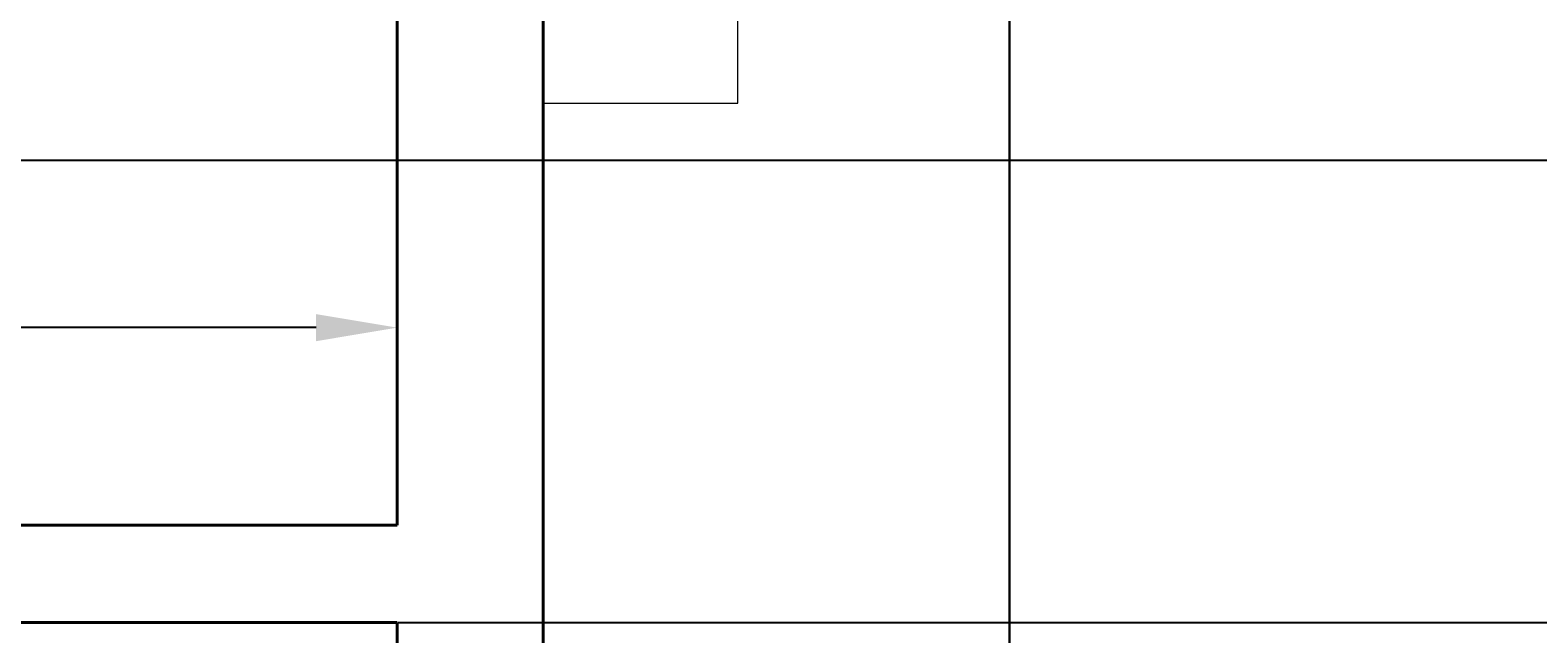
# Model space of a CAD drawing. Units: inches. Extents: x -301 to 715, y -607 to 364.
# Tile 120 of 141: x 101 to 194, y 192 to 230. Entities that reach past the tile are written whole.
import ezdxf

# ---------------------------------------------------------------- set-up
doc = ezdxf.new("R2010")
doc.units = ezdxf.units.IN
doc.header["$MEASUREMENT"] = 0
doc.linetypes.add('ACAD_ISO02W100', pattern=[15, 12, -3])
for name, color, linetype, lineweight in [('A-ANNO-DIMS', 2, 'Continuous', 18), ('A-GLAZ-OVHD', 2, 'ACAD_ISO02W100', 18), ('A-WALL', 3, 'Continuous', 40)]:
    doc.layers.add(name, color=color, linetype=linetype, lineweight=lineweight)
doc.styles.get("Standard").update_dxf_attribs({"font": 'arial.ttf'})
doc.dimstyles.get("Standard").update_dxf_attribs({"dimtxt": 0.18, "dimasz": 0.18, "dimexe": 0.18, "dimexo": 0.0625, "dimgap": 0.09, "dimtad": 0, "dimtih": 1, "dimtoh": 1, "dimdec": 1, "dimzin": 0, "dimdsep": 46, "dimlunit": 4, "dimtxsty": 'Standard', "dimcen": 0.09, "dimclrd": 3, "dimclre": 4, "dimclrt": 6, "dimadec": 0, "dimazin": 0, "dimtfac": 1, "dimtdec": 1, "dimtofl": 0, "dimtmove": 0, "dimatfit": 3, "dimfxl": 1, "dimtfill": 2, "dimtfillclr": 51, "dimtolj": 1, "dimtzin": 0, "dimarcsym": 0})

# ---------------------------------------------------------------- blocks, each defined once
blk = doc.blocks.new('*D50')
at = {"layer": 'A-ANNO-DIMS', "color": 0, "lineweight": -2, "transparency": 16777216}
for p, q in [((15.897, 199.83), (15.897, 211.535)), ((20.897, 211.355), (68.426, 211.355)), ((118.897, 211.355), (71.367, 211.355)), ((123.897, 199.245), (123.897, 211.535))]:
    blk.add_line(p, q, dxfattribs=at)
at = {"layer": 'A-ANNO-DIMS', "color": 0, "transparency": 16777216}
for points in [[(20.897, 212.188), (20.897, 210.521), (15.897, 211.355)], [(118.897, 212.188), (118.897, 210.521), (123.897, 211.355)]]:
    blk.add_solid(points, dxfattribs=at)
at = {"layer": 'Defpoints', "color": 0, "transparency": 16777216}
for p in [(15.897, 211.355), (15.897, 199.767), (123.897, 199.182)]:
    blk.add_point(p, dxfattribs=at)
at = {"layer": 'A-ANNO-DIMS', "color": 0, "transparency": 16777216, "insert": (69.897, 211.355), "char_height": 3, "attachment_point": 5, "bg_fill": 1, "box_fill_scale": 1.25, "bg_fill_color": 51, "bg_fill_transparency": 0}
blk.add_mtext("\\A1;9'", dxfattribs=at)
blk = doc.blocks.new('WIN-SHADE-50')
at = {"ltscale": 1.5}
for p, q in [((0, 0), (0, 12)), ((50, 12), (0, 12)), ((50, 0), (50, 12)), ((5, 0), (0, 0)), ((45, 0), (50, 0))]:
    blk.add_line(p, q, dxfattribs=at)
blk = doc.blocks.new('*D153')
at = {"layer": 'A-ANNO-DIMS', "color": 4, "lineweight": -2, "transparency": 16777216}
for p, q in [((132.959, 310.182), (233.659, 310.182)), ((123.959, 193.182), (233.659, 193.182))]:
    blk.add_line(p, q, dxfattribs=at)
at = {"layer": 'A-ANNO-DIMS', "color": 3, "lineweight": -2, "transparency": 16777216}
for p, q in [((233.479, 310.002), (233.479, 251.864)), ((233.479, 193.362), (233.479, 251.5))]:
    blk.add_line(p, q, dxfattribs=at)
at = {"layer": 'A-ANNO-DIMS', "color": 3, "transparency": 16777216}
for points in [[(233.449, 310.002), (233.509, 310.002), (233.479, 310.182)], [(233.449, 193.362), (233.509, 193.362), (233.479, 193.182)]]:
    blk.add_solid(points, dxfattribs=at)
at = {"layer": 'Defpoints', "color": 0, "transparency": 16777216}
for p in [(132.897, 310.182), (123.897, 193.182), (233.479, 193.182)]:
    blk.add_point(p, dxfattribs=at)
at = {"layer": 'A-ANNO-DIMS', "color": 6, "transparency": 16777216, "insert": (233.479, 251.682), "char_height": 0.18, "attachment_point": 5, "bg_fill": 1, "box_fill_scale": 1.25, "bg_fill_color": 51, "bg_fill_transparency": 0}
blk.add_mtext('\\A1;9\'-9"', dxfattribs=at)
blk = doc.blocks.new('*D157')
at = {"layer": 'A-ANNO-DIMS', "color": 4, "lineweight": -2, "transparency": 16777216}
for p, q in [((-50.541, 261.432), (233.659, 261.432)), ((-50.541, 221.682), (233.659, 221.682))]:
    blk.add_line(p, q, dxfattribs=at)
at = {"layer": 'A-ANNO-DIMS', "color": 3, "lineweight": -2, "transparency": 16777216}
for p, q in [((233.479, 261.252), (233.479, 241.739)), ((233.479, 221.862), (233.479, 241.375))]:
    blk.add_line(p, q, dxfattribs=at)
at = {"layer": 'A-ANNO-DIMS', "color": 3, "transparency": 16777216}
for points in [[(233.449, 261.252), (233.509, 261.252), (233.479, 261.432)], [(233.449, 221.862), (233.509, 221.862), (233.479, 221.682)]]:
    blk.add_solid(points, dxfattribs=at)
at = {"layer": 'Defpoints', "color": 0, "transparency": 16777216}
for p in [(-50.603, 261.432), (233.479, 261.432), (-50.603, 221.682)]:
    blk.add_point(p, dxfattribs=at)
at = {"layer": 'A-ANNO-DIMS', "color": 6, "transparency": 16777216, "insert": (233.479, 241.557), "char_height": 0.18, "attachment_point": 5, "bg_fill": 1, "box_fill_scale": 1.25, "bg_fill_color": 51, "bg_fill_transparency": 0}
blk.add_mtext('\\A1;3\'-4"', dxfattribs=at)
blk = doc.blocks.new('*D162')
at = {"layer": 'A-ANNO-DIMS', "color": 4, "lineweight": -2, "transparency": 16777216}
for p, q in [((222.328, 320.182), (161.439, 320.182)), ((222.328, -233.818), (161.439, -233.818))]:
    blk.add_line(p, q, dxfattribs=at)
at = {"layer": 'A-ANNO-DIMS', "color": 3, "lineweight": -2, "transparency": 16777216}
for p, q in [((161.619, 320.002), (161.619, 43.364)), ((161.619, -233.638), (161.619, 43))]:
    blk.add_line(p, q, dxfattribs=at)
at = {"layer": 'A-ANNO-DIMS', "color": 3, "transparency": 16777216}
for points in [[(161.589, 320.002), (161.649, 320.002), (161.619, 320.182)], [(161.589, -233.638), (161.649, -233.638), (161.619, -233.818)]]:
    blk.add_solid(points, dxfattribs=at)
at = {"layer": 'Defpoints', "color": 0, "transparency": 16777216}
for p in [(161.619, 320.182), (222.39, 320.182), (222.39, -233.818)]:
    blk.add_point(p, dxfattribs=at)
at = {"layer": 'A-ANNO-DIMS', "color": 6, "transparency": 16777216, "insert": (161.619, 43.182), "char_height": 0.18, "attachment_point": 5, "bg_fill": 1, "box_fill_scale": 1.25, "bg_fill_color": 51, "bg_fill_transparency": 0}
blk.add_mtext('\\A1;46\'-2"', dxfattribs=at)
blk = doc.blocks.new('*D170')
at = {"layer": 'A-ANNO-DIMS', "color": 4, "lineweight": -2, "transparency": 16777216}
for p, q in [((222.328, 291.182), (161.439, 291.182)), ((222.328, 183.182), (161.439, 183.182))]:
    blk.add_line(p, q, dxfattribs=at)
at = {"layer": 'A-ANNO-DIMS', "color": 3, "lineweight": -2, "transparency": 16777216}
for p, q in [((161.619, 291.002), (161.619, 237.364)), ((161.619, 183.362), (161.619, 237))]:
    blk.add_line(p, q, dxfattribs=at)
at = {"layer": 'A-ANNO-DIMS', "color": 3, "transparency": 16777216}
for points in [[(161.589, 291.002), (161.649, 291.002), (161.619, 291.182)], [(161.589, 183.362), (161.649, 183.362), (161.619, 183.182)]]:
    blk.add_solid(points, dxfattribs=at)
at = {"layer": 'Defpoints', "color": 0, "transparency": 16777216}
for p in [(161.619, 291.182), (222.39, 291.182), (222.39, 183.182)]:
    blk.add_point(p, dxfattribs=at)
at = {"layer": 'A-ANNO-DIMS', "color": 6, "transparency": 16777216, "insert": (161.619, 237.182), "char_height": 0.18, "attachment_point": 5, "bg_fill": 1, "box_fill_scale": 1.25, "bg_fill_color": 51, "bg_fill_transparency": 0}
blk.add_mtext('\\A1;9\'-0"', dxfattribs=at)

msp = doc.modelspace()

# ---------------------------------------------------------------- linework, layer by layer
at = {"layer": 'A-WALL'}
for p, q in [((132.897, 199.182), (132.897, 310.182)), ((123.897, 199.182), (123.897, 301.182)), ((123.897, 199.182), (55.897, 199.182)), ((132.897, -9.818), (132.897, 199.182)), ((123.897, 193.182), (55.897, 193.182)), ((123.897, -9.818), (123.897, 193.182))]:
    msp.add_line(p, q, dxfattribs=at)

# ---------------------------------------------------------------- block references
at = {"layer": 'A-GLAZ-OVHD', "rotation": 270.0000000000002}
msp.add_blockref('WIN-SHADE-50', (132.896, 275.182), dxfattribs=at)

# ---------------------------------------------------------------- dimensions: what is measured, and where the dimension line sits
at = {"layer": 'A-ANNO-DIMS'}
for base, p1, p2, picture, middle in [((161.619, 320.182), (222.39, -233.818), (222.39, 320.182), '*D162', (161.619, 43.182)), ((233.479, 193.182), (132.897, 310.182), (123.897, 193.182), '*D153', (233.479, 251.682)), ((161.619, 291.182), (222.39, 183.182), (222.39, 291.182), '*D170', (161.619, 237.182)), ((233.479242, 261.43233), (-50.603288, 221.68233), (-50.603288, 261.43233), '*D157', (233.479242, 241.55733))]:
    dim = msp.add_linear_dim(base=base, p1=p1, p2=p2, angle=90, dimstyle='Standard', override={"dimdec": 1, "dimlfac": 1, "dimrnd": 0, "dimzin": 1, "dimdsep": 46, "dimlunit": 4, "dimfrac": 2}, dxfattribs=at)
    dim.commit()
    dim.dimension.update_dxf_attribs({"geometry": picture, "text_midpoint": middle})
dim = msp.add_linear_dim(base=(15.897, 211.355), p1=(123.897, 199.182), p2=(15.897, 199.767), dimstyle='Standard', override={"dimtxt": 3, "dimasz": 5, "dimclrd": 0, "dimclre": 0, "dimclrt": 0}, dxfattribs=at)
dim.commit()
dim.dimension.update_dxf_attribs({"geometry": '*D50', "text_midpoint": (69.897, 211.355)})

doc.saveas('drawing.dxf')
